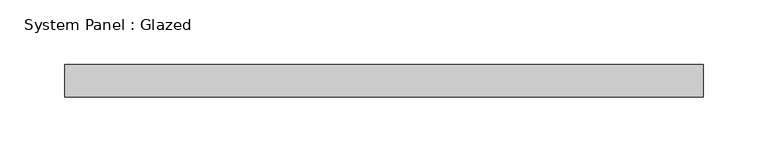
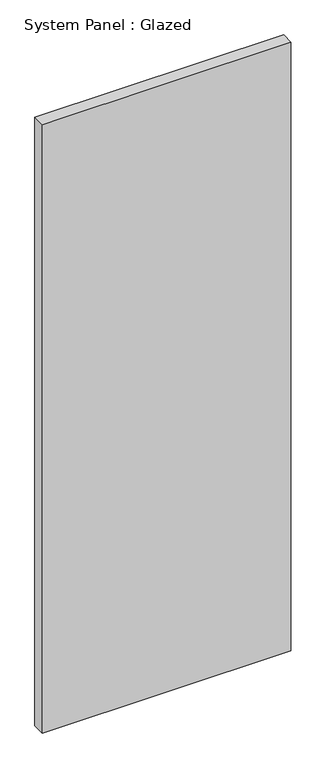
"""IFC4 building model written with IfcOpenShell, lengths in millimetres: plate geometry, System Panel : Glazed."""

from ifc_helpers import new_model, si_unit, origin, origin_with_axes, place, context, project, spatial, polyline, outline, extrude, source, transform, mapped, element, save


def system_panel_glazed_4ceb7c04(model_context):
    return source(origin(), model_context, "Body", "SweptSolid", [
        extrude(outline(polyline([(247.65, 19.05), (-247.65, 19.05), (-247.65, 44.45), (247.65, 44.45), (247.65, 19.05)])), origin_with_axes(), (0.0, 0.0, 1.0), 1281.187673),
    ])


if __name__ == "__main__":
    model = new_model("IFC4")
    model_context = context("Model", 3, world=origin())
    ifc_project = project(units=[si_unit("LENGTHUNIT", "METRE", prefix="MILLI")], contexts=[model_context])
    site = spatial("IfcSite", under=ifc_project)
    building = spatial("IfcBuilding", under=site)
    placement = place(None, origin())
    system_panel_glazed_shape = system_panel_glazed_4ceb7c04(model_context)
    element("IfcPlate", 1, ObjectType="System Panel : Glazed", at=placement, inside=building, context=model_context, shape_type="MappedRepresentation", body=[
        mapped(system_panel_glazed_shape, transform((0.0, 0.0, 0.0), x_axis=(1.0, 0.0, 0.0), y_axis=(0.0, 1.0, 0.0), z_axis=(0.0, 0.0, 1.0))),
    ])
    save(model, "model.ifc")

# Revit data of these elements
# Type "System Panel : Glazed"
#   Construction Type Id = "GSP4R"
#   Analytic Construction = "1/8 in Pilkington single glazing"
#   Visual Light Transmittance = 0.9
#   Solar Heat Gain Coefficient = 0.86
#   Heat Transfer Coefficient (U) = 1.18115 BTU/(h·ft²·°F)
#   Define Thermal Properties by = 1
# Element 1 (IfcPlate, "System Panel : Glazed")
#   Materials on its faces: "Glass"
# Materials
#   "Glass": class "Glass", colour RGB 0 128 192, transparency 0.75, Description = "Soda Lime Glass", Cost = 0
